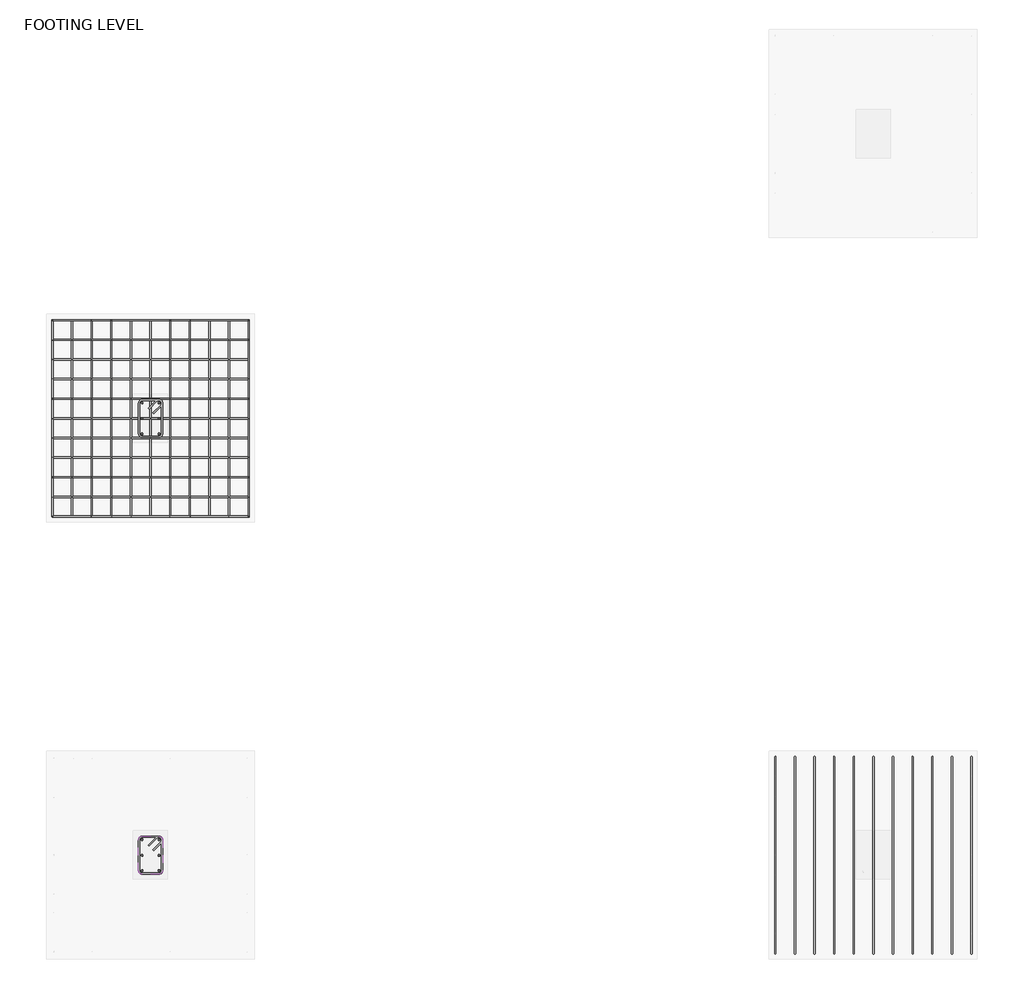
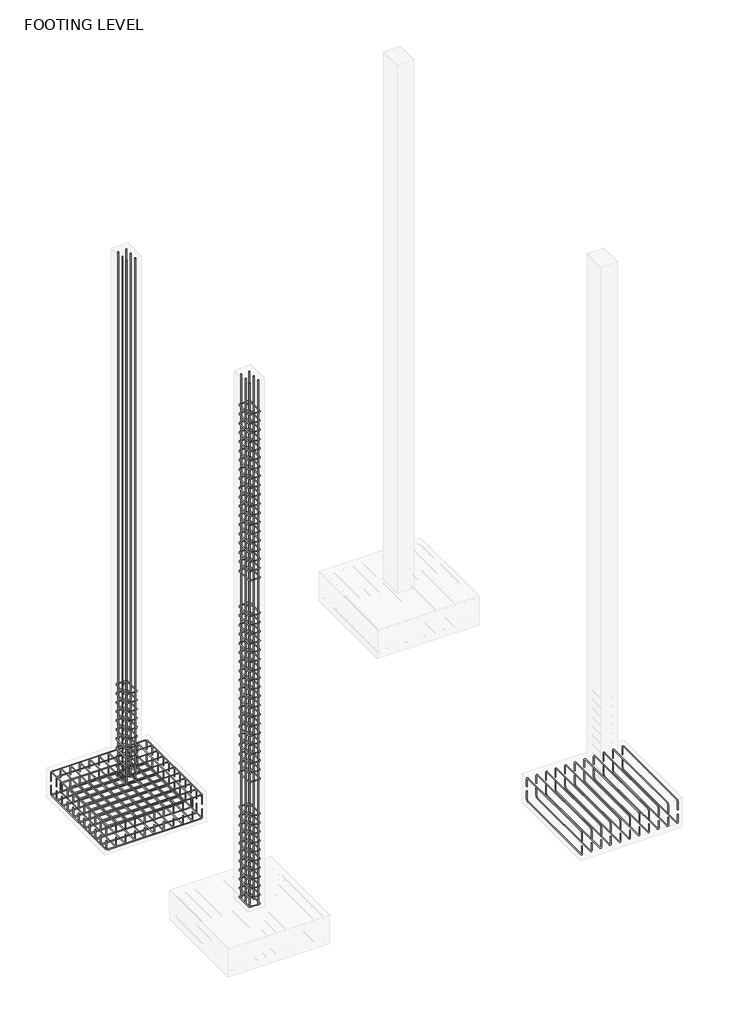
# One storey, part 3 of 9: 22 reinforcing bars.
"""IFC4 building model written with IfcOpenShell, lengths in millimetres."""

from ifc_helpers import new_model, si_unit, point, frame, origin, place, context, project, spatial, polyline, circle_curve, trimmed, segment, composite_curve, source, transform, mapped, element, save
from ifc_brep_helpers import swept_disk

model = new_model("IFC4")

# Units and contexts
model_context = context("Model", 3, world=origin())
ifc_project = project(units=[si_unit("LENGTHUNIT", "METRE", prefix="MILLI")], contexts=[model_context])

# Site, building, storey
site = spatial("IfcSite", under=ifc_project)
building = spatial("IfcBuilding", under=site)
storey = spatial("IfcBuildingStorey", under=building, Name="FOOTING LEVEL", Elevation=-1981.2)

# Reinforcing bars
placement = place(None, origin())
reinforcing_bar_shape = source(origin(), model_context, "Body", "SolidModel", [
    swept_disk(composite_curve([segment(polyline([(-2537.1816189, -3042.2841598, -2171.7), (-2537.1816189, -3042.2841598, -2057.4)]), True, "CONTINUOUS"), segment(trimmed(circle_curve(frame((-2537.1816189, -3075.6216598, -2057.4), z_axis=(1.0, 0.0, 0.0), x_axis=(0.0, 33.33750000000009, 0.0)), 33.3375), [point((-2537.1816189, -3042.2841598, -2057.4))], [point((-2537.1816189, -3075.6216598, -2024.0625))], True, "CARTESIAN"), True, "CONTINUOUS"), segment(polyline([(-2537.1816189, -3075.6216598, -2024.0625), (-2537.1816189, -4447.2216598, -2024.0625)]), True, "CONTINUOUS"), segment(trimmed(circle_curve(frame((-2537.1816189, -4447.2216598, -2057.4), z_axis=(1.0, 0.0, 0.0), x_axis=(0.0, 0.0, 33.33750000000009)), 33.3375), [point((-2537.1816189, -4447.2216598, -2024.0625))], [point((-2537.1816189, -4480.5591598, -2057.4))], True, "CARTESIAN"), True, "CONTINUOUS"), segment(polyline([(-2537.1816189, -4480.5591598, -2057.4), (-2537.1816189, -4480.5591598, -2171.7)]), True, "CONTINUOUS")], self_intersect=False), 4.7625),
])
element("IfcReinforcingBar", 1, at=placement, inside=storey, context=model_context, shape_type="MappedRepresentation", body=[
    mapped(reinforcing_bar_shape, transform((0.0, 0.0, 0.0), x_axis=(1.0, 0.0, 0.0), y_axis=(0.0, 1.0, 0.0), z_axis=(0.0, 0.0, 1.0))),
    mapped(reinforcing_bar_shape, transform((-143.8275, 0.0, 0.0), x_axis=(1.0, 0.0, 0.0), y_axis=(0.0, 1.0, 0.0), z_axis=(0.0, 0.0, 1.0))),
    mapped(reinforcing_bar_shape, transform((-287.655, 0.0, 0.0), x_axis=(1.0, 0.0, 0.0), y_axis=(0.0, 1.0, 0.0), z_axis=(0.0, 0.0, 1.0))),
    mapped(reinforcing_bar_shape, transform((-431.4825, 0.0, 0.0), x_axis=(1.0, 0.0, 0.0), y_axis=(0.0, 1.0, 0.0), z_axis=(0.0, 0.0, 1.0))),
    mapped(reinforcing_bar_shape, transform((-575.31, 0.0, 0.0), x_axis=(1.0, 0.0, 0.0), y_axis=(0.0, 1.0, 0.0), z_axis=(0.0, 0.0, 1.0))),
    mapped(reinforcing_bar_shape, transform((-719.1375, 0.0, 0.0), x_axis=(1.0, 0.0, 0.0), y_axis=(0.0, 1.0, 0.0), z_axis=(0.0, 0.0, 1.0))),
    mapped(reinforcing_bar_shape, transform((-862.965, 0.0, 0.0), x_axis=(1.0, 0.0, 0.0), y_axis=(0.0, 1.0, 0.0), z_axis=(0.0, 0.0, 1.0))),
    mapped(reinforcing_bar_shape, transform((-1006.7925, 0.0, 0.0), x_axis=(1.0, 0.0, 0.0), y_axis=(0.0, 1.0, 0.0), z_axis=(0.0, 0.0, 1.0))),
    mapped(reinforcing_bar_shape, transform((-1150.62, 0.0, 0.0), x_axis=(1.0, 0.0, 0.0), y_axis=(0.0, 1.0, 0.0), z_axis=(0.0, 0.0, 1.0))),
    mapped(reinforcing_bar_shape, transform((-1294.4475, 0.0, 0.0), x_axis=(1.0, 0.0, 0.0), y_axis=(0.0, 1.0, 0.0), z_axis=(0.0, 0.0, 1.0))),
    mapped(reinforcing_bar_shape, transform((-1438.275, 0.0, 0.0), x_axis=(1.0, 0.0, 0.0), y_axis=(0.0, 1.0, 0.0), z_axis=(0.0, 0.0, 1.0))),
])
reinforcing_bar_2_shape = source(origin(), model_context, "Body", "SolidModel", [
    swept_disk(composite_curve([segment(polyline([(-2537.1816189, -4480.5591598, -2247.9), (-2537.1816189, -4480.5591598, -2362.2)]), True, "CONTINUOUS"), segment(trimmed(circle_curve(frame((-2537.1816189, -4447.2216598, -2362.2), z_axis=(1.0, 0.0, 0.0), x_axis=(0.0, -33.337499999999636, 0.0)), 33.3375), [point((-2537.1816189, -4480.5591598, -2362.2))], [point((-2537.1816189, -4447.2216598, -2395.5375))], True, "CARTESIAN"), True, "CONTINUOUS"), segment(polyline([(-2537.1816189, -4447.2216598, -2395.5375), (-2537.1816189, -3075.6216598, -2395.5375)]), True, "CONTINUOUS"), segment(trimmed(circle_curve(frame((-2537.1816189, -3075.6216598, -2362.2), z_axis=(1.0, 0.0, 0.0), x_axis=(0.0, 0.0, -33.33750000000009)), 33.3375), [point((-2537.1816189, -3075.6216598, -2395.5375))], [point((-2537.1816189, -3042.2841598, -2362.2))], True, "CARTESIAN"), True, "CONTINUOUS"), segment(polyline([(-2537.1816189, -3042.2841598, -2362.2), (-2537.1816189, -3042.2841598, -2247.9)]), True, "CONTINUOUS")], self_intersect=False), 4.7625),
])
element("IfcReinforcingBar", 2, at=placement, inside=storey, context=model_context, shape_type="MappedRepresentation", body=[
    mapped(reinforcing_bar_2_shape, transform((0.0, 0.0, 0.0), x_axis=(1.0, 0.0, 0.0), y_axis=(0.0, 1.0, 0.0), z_axis=(0.0, 0.0, 1.0))),
    mapped(reinforcing_bar_2_shape, transform((-143.8275, 0.0, 0.0), x_axis=(1.0, 0.0, 0.0), y_axis=(0.0, 1.0, 0.0), z_axis=(0.0, 0.0, 1.0))),
    mapped(reinforcing_bar_2_shape, transform((-287.655, 0.0, 0.0), x_axis=(1.0, 0.0, 0.0), y_axis=(0.0, 1.0, 0.0), z_axis=(0.0, 0.0, 1.0))),
    mapped(reinforcing_bar_2_shape, transform((-431.4825, 0.0, 0.0), x_axis=(1.0, 0.0, 0.0), y_axis=(0.0, 1.0, 0.0), z_axis=(0.0, 0.0, 1.0))),
    mapped(reinforcing_bar_2_shape, transform((-575.31, 0.0, 0.0), x_axis=(1.0, 0.0, 0.0), y_axis=(0.0, 1.0, 0.0), z_axis=(0.0, 0.0, 1.0))),
    mapped(reinforcing_bar_2_shape, transform((-719.1375, 0.0, 0.0), x_axis=(1.0, 0.0, 0.0), y_axis=(0.0, 1.0, 0.0), z_axis=(0.0, 0.0, 1.0))),
    mapped(reinforcing_bar_2_shape, transform((-862.965, 0.0, 0.0), x_axis=(1.0, 0.0, 0.0), y_axis=(0.0, 1.0, 0.0), z_axis=(0.0, 0.0, 1.0))),
    mapped(reinforcing_bar_2_shape, transform((-1006.7925, 0.0, 0.0), x_axis=(1.0, 0.0, 0.0), y_axis=(0.0, 1.0, 0.0), z_axis=(0.0, 0.0, 1.0))),
    mapped(reinforcing_bar_2_shape, transform((-1150.62, 0.0, 0.0), x_axis=(1.0, 0.0, 0.0), y_axis=(0.0, 1.0, 0.0), z_axis=(0.0, 0.0, 1.0))),
    mapped(reinforcing_bar_2_shape, transform((-1294.4475, 0.0, 0.0), x_axis=(1.0, 0.0, 0.0), y_axis=(0.0, 1.0, 0.0), z_axis=(0.0, 0.0, 1.0))),
    mapped(reinforcing_bar_2_shape, transform((-1438.275, 0.0, 0.0), x_axis=(1.0, 0.0, 0.0), y_axis=(0.0, 1.0, 0.0), z_axis=(0.0, 0.0, 1.0))),
])
reinforcing_bar_3_shape = source(origin(), model_context, "Body", "SolidModel", [
    swept_disk(composite_curve([segment(polyline([(-7832.9458659, 158.1158402, -2171.7), (-7832.9458659, 158.1158402, -2057.4)]), True, "CONTINUOUS"), segment(trimmed(circle_curve(frame((-7832.9458659, 124.7783402, -2057.4), z_axis=(1.0, 0.0, 0.0), x_axis=(0.0, 33.337500000000006, 0.0)), 33.3375), [point((-7832.9458659, 158.1158402, -2057.4))], [point((-7832.9458659, 124.7783402, -2024.0625))], True, "CARTESIAN"), True, "CONTINUOUS"), segment(polyline([(-7832.9458659, 124.7783402, -2024.0625), (-7832.9458659, -1246.8216598, -2024.0625)]), True, "CONTINUOUS"), segment(trimmed(circle_curve(frame((-7832.9458659, -1246.8216598, -2057.4), z_axis=(1.0, 0.0, 0.0), x_axis=(0.0, 0.0, 33.33750000000009)), 33.3375), [point((-7832.9458659, -1246.8216598, -2024.0625))], [point((-7832.9458659, -1280.1591598, -2057.4))], True, "CARTESIAN"), True, "CONTINUOUS"), segment(polyline([(-7832.9458659, -1280.1591598, -2057.4), (-7832.9458659, -1280.1591598, -2171.7)]), True, "CONTINUOUS")], self_intersect=False), 4.7625),
])
element("IfcReinforcingBar", 3, at=placement, inside=storey, context=model_context, shape_type="MappedRepresentation", body=[
    mapped(reinforcing_bar_3_shape, transform((0.0, 0.0, 0.0), x_axis=(1.0, 0.0, 0.0), y_axis=(0.0, 1.0, 0.0), z_axis=(0.0, 0.0, 1.0))),
    mapped(reinforcing_bar_3_shape, transform((-143.8275, 0.0, 0.0), x_axis=(1.0, 0.0, 0.0), y_axis=(0.0, 1.0, 0.0), z_axis=(0.0, 0.0, 1.0))),
    mapped(reinforcing_bar_3_shape, transform((-287.655, 0.0, 0.0), x_axis=(1.0, 0.0, 0.0), y_axis=(0.0, 1.0, 0.0), z_axis=(0.0, 0.0, 1.0))),
    mapped(reinforcing_bar_3_shape, transform((-431.4825, 0.0, 0.0), x_axis=(1.0, 0.0, 0.0), y_axis=(0.0, 1.0, 0.0), z_axis=(0.0, 0.0, 1.0))),
    mapped(reinforcing_bar_3_shape, transform((-575.31, 0.0, 0.0), x_axis=(1.0, 0.0, 0.0), y_axis=(0.0, 1.0, 0.0), z_axis=(0.0, 0.0, 1.0))),
    mapped(reinforcing_bar_3_shape, transform((-719.1375, 0.0, 0.0), x_axis=(1.0, 0.0, 0.0), y_axis=(0.0, 1.0, 0.0), z_axis=(0.0, 0.0, 1.0))),
    mapped(reinforcing_bar_3_shape, transform((-862.965, 0.0, 0.0), x_axis=(1.0, 0.0, 0.0), y_axis=(0.0, 1.0, 0.0), z_axis=(0.0, 0.0, 1.0))),
    mapped(reinforcing_bar_3_shape, transform((-1006.7925, 0.0, 0.0), x_axis=(1.0, 0.0, 0.0), y_axis=(0.0, 1.0, 0.0), z_axis=(0.0, 0.0, 1.0))),
    mapped(reinforcing_bar_3_shape, transform((-1150.62, 0.0, 0.0), x_axis=(1.0, 0.0, 0.0), y_axis=(0.0, 1.0, 0.0), z_axis=(0.0, 0.0, 1.0))),
    mapped(reinforcing_bar_3_shape, transform((-1294.4475, 0.0, 0.0), x_axis=(1.0, 0.0, 0.0), y_axis=(0.0, 1.0, 0.0), z_axis=(0.0, 0.0, 1.0))),
    mapped(reinforcing_bar_3_shape, transform((-1438.275, 0.0, 0.0), x_axis=(1.0, 0.0, 0.0), y_axis=(0.0, 1.0, 0.0), z_axis=(0.0, 0.0, 1.0))),
])
reinforcing_bar_4_shape = source(origin(), model_context, "Body", "SolidModel", [
    swept_disk(composite_curve([segment(polyline([(-7832.9458659, -1280.1591598, -2247.9), (-7832.9458659, -1280.1591598, -2362.2)]), True, "CONTINUOUS"), segment(trimmed(circle_curve(frame((-7832.9458659, -1246.8216598, -2362.2), z_axis=(1.0, 0.0, 0.0), x_axis=(0.0, -33.33750000000009, 0.0)), 33.3375), [point((-7832.9458659, -1280.1591598, -2362.2))], [point((-7832.9458659, -1246.8216598, -2395.5375))], True, "CARTESIAN"), True, "CONTINUOUS"), segment(polyline([(-7832.9458659, -1246.8216598, -2395.5375), (-7832.9458659, 124.7783402, -2395.5375)]), True, "CONTINUOUS"), segment(trimmed(circle_curve(frame((-7832.9458659, 124.7783402, -2362.2), z_axis=(1.0, 0.0, 0.0), x_axis=(0.0, 0.0, -33.33750000000009)), 33.3375), [point((-7832.9458659, 124.7783402, -2395.5375))], [point((-7832.9458659, 158.1158402, -2362.2))], True, "CARTESIAN"), True, "CONTINUOUS"), segment(polyline([(-7832.9458659, 158.1158402, -2362.2), (-7832.9458659, 158.1158402, -2247.9)]), True, "CONTINUOUS")], self_intersect=False), 4.7625),
])
element("IfcReinforcingBar", 4, at=placement, inside=storey, context=model_context, shape_type="MappedRepresentation", body=[
    mapped(reinforcing_bar_4_shape, transform((0.0, 0.0, 0.0), x_axis=(1.0, 0.0, 0.0), y_axis=(0.0, 1.0, 0.0), z_axis=(0.0, 0.0, 1.0))),
    mapped(reinforcing_bar_4_shape, transform((-143.8275, 0.0, 0.0), x_axis=(1.0, 0.0, 0.0), y_axis=(0.0, 1.0, 0.0), z_axis=(0.0, 0.0, 1.0))),
    mapped(reinforcing_bar_4_shape, transform((-287.655, 0.0, 0.0), x_axis=(1.0, 0.0, 0.0), y_axis=(0.0, 1.0, 0.0), z_axis=(0.0, 0.0, 1.0))),
    mapped(reinforcing_bar_4_shape, transform((-431.4825, 0.0, 0.0), x_axis=(1.0, 0.0, 0.0), y_axis=(0.0, 1.0, 0.0), z_axis=(0.0, 0.0, 1.0))),
    mapped(reinforcing_bar_4_shape, transform((-575.31, 0.0, 0.0), x_axis=(1.0, 0.0, 0.0), y_axis=(0.0, 1.0, 0.0), z_axis=(0.0, 0.0, 1.0))),
    mapped(reinforcing_bar_4_shape, transform((-719.1375, 0.0, 0.0), x_axis=(1.0, 0.0, 0.0), y_axis=(0.0, 1.0, 0.0), z_axis=(0.0, 0.0, 1.0))),
    mapped(reinforcing_bar_4_shape, transform((-862.965, 0.0, 0.0), x_axis=(1.0, 0.0, 0.0), y_axis=(0.0, 1.0, 0.0), z_axis=(0.0, 0.0, 1.0))),
    mapped(reinforcing_bar_4_shape, transform((-1006.7925, 0.0, 0.0), x_axis=(1.0, 0.0, 0.0), y_axis=(0.0, 1.0, 0.0), z_axis=(0.0, 0.0, 1.0))),
    mapped(reinforcing_bar_4_shape, transform((-1150.62, 0.0, 0.0), x_axis=(1.0, 0.0, 0.0), y_axis=(0.0, 1.0, 0.0), z_axis=(0.0, 0.0, 1.0))),
    mapped(reinforcing_bar_4_shape, transform((-1294.4475, 0.0, 0.0), x_axis=(1.0, 0.0, 0.0), y_axis=(0.0, 1.0, 0.0), z_axis=(0.0, 0.0, 1.0))),
    mapped(reinforcing_bar_4_shape, transform((-1438.275, 0.0, 0.0), x_axis=(1.0, 0.0, 0.0), y_axis=(0.0, 1.0, 0.0), z_axis=(0.0, 0.0, 1.0))),
])
reinforcing_bar_5_shape = source(origin(), model_context, "Body", "SolidModel", [
    swept_disk(composite_curve([segment(polyline([(-9271.2208659, 158.1158402, -2171.7), (-9271.2208659, 158.1158402, -2057.4)]), True, "CONTINUOUS"), segment(trimmed(circle_curve(frame((-9237.8833659, 158.1158402, -2057.4), z_axis=(0.0, 1.0, 0.0), x_axis=(-33.337500000001455, 0.0, 0.0)), 33.3375), [point((-9271.2208659, 158.1158402, -2057.4))], [point((-9237.8833659, 158.1158402, -2024.0625))], True, "CARTESIAN"), True, "CONTINUOUS"), segment(polyline([(-9237.8833659, 158.1158402, -2024.0625), (-7866.2833659, 158.1158402, -2024.0625)]), True, "CONTINUOUS"), segment(trimmed(circle_curve(frame((-7866.2833659, 158.1158402, -2057.4), z_axis=(0.0, 1.0, 0.0), x_axis=(0.0, 0.0, 33.33750000000009)), 33.3375), [point((-7866.2833659, 158.1158402, -2024.0625))], [point((-7832.9458659, 158.1158402, -2057.4))], True, "CARTESIAN"), True, "CONTINUOUS"), segment(polyline([(-7832.9458659, 158.1158402, -2057.4), (-7832.9458659, 158.1158402, -2171.7)]), True, "CONTINUOUS")], self_intersect=False), 4.7625),
])
element("IfcReinforcingBar", 5, at=placement, inside=storey, context=model_context, shape_type="MappedRepresentation", body=[
    mapped(reinforcing_bar_5_shape, transform((0.0, 0.0, 0.0), x_axis=(1.0, 0.0, 0.0), y_axis=(0.0, 1.0, 0.0), z_axis=(0.0, 0.0, 1.0))),
    mapped(reinforcing_bar_5_shape, transform((0.0, -143.8275, 0.0), x_axis=(1.0, 0.0, 0.0), y_axis=(0.0, 1.0, 0.0), z_axis=(0.0, 0.0, 1.0))),
    mapped(reinforcing_bar_5_shape, transform((0.0, -287.655, 0.0), x_axis=(1.0, 0.0, 0.0), y_axis=(0.0, 1.0, 0.0), z_axis=(0.0, 0.0, 1.0))),
    mapped(reinforcing_bar_5_shape, transform((0.0, -431.4825, 0.0), x_axis=(1.0, 0.0, 0.0), y_axis=(0.0, 1.0, 0.0), z_axis=(0.0, 0.0, 1.0))),
    mapped(reinforcing_bar_5_shape, transform((0.0, -575.31, 0.0), x_axis=(1.0, 0.0, 0.0), y_axis=(0.0, 1.0, 0.0), z_axis=(0.0, 0.0, 1.0))),
    mapped(reinforcing_bar_5_shape, transform((0.0, -719.1375, 0.0), x_axis=(1.0, 0.0, 0.0), y_axis=(0.0, 1.0, 0.0), z_axis=(0.0, 0.0, 1.0))),
    mapped(reinforcing_bar_5_shape, transform((0.0, -862.965, 0.0), x_axis=(1.0, 0.0, 0.0), y_axis=(0.0, 1.0, 0.0), z_axis=(0.0, 0.0, 1.0))),
    mapped(reinforcing_bar_5_shape, transform((0.0, -1006.7925, 0.0), x_axis=(1.0, 0.0, 0.0), y_axis=(0.0, 1.0, 0.0), z_axis=(0.0, 0.0, 1.0))),
    mapped(reinforcing_bar_5_shape, transform((0.0, -1150.62, 0.0), x_axis=(1.0, 0.0, 0.0), y_axis=(0.0, 1.0, 0.0), z_axis=(0.0, 0.0, 1.0))),
    mapped(reinforcing_bar_5_shape, transform((0.0, -1294.4475, 0.0), x_axis=(1.0, 0.0, 0.0), y_axis=(0.0, 1.0, 0.0), z_axis=(0.0, 0.0, 1.0))),
    mapped(reinforcing_bar_5_shape, transform((0.0, -1438.275, 0.0), x_axis=(1.0, 0.0, 0.0), y_axis=(0.0, 1.0, 0.0), z_axis=(0.0, 0.0, 1.0))),
])
reinforcing_bar_6_shape = source(origin(), model_context, "Body", "SolidModel", [
    swept_disk(composite_curve([segment(polyline([(-9271.2208659, -1280.1591598, -2247.9), (-9271.2208659, -1280.1591598, -2362.2)]), True, "CONTINUOUS"), segment(trimmed(circle_curve(frame((-9237.8833659, -1280.1591598, -2362.2), z_axis=(0.0, -1.0, 0.0), x_axis=(-33.337500000001455, 0.0, 0.0)), 33.3375), [point((-9271.2208659, -1280.1591598, -2362.2))], [point((-9237.8833659, -1280.1591598, -2395.5375))], True, "CARTESIAN"), True, "CONTINUOUS"), segment(polyline([(-9237.8833659, -1280.1591598, -2395.5375), (-7866.2833659, -1280.1591598, -2395.5375)]), True, "CONTINUOUS"), segment(trimmed(circle_curve(frame((-7866.2833659, -1280.1591598, -2362.2), z_axis=(0.0, -1.0, 0.0), x_axis=(0.0, 0.0, -33.33750000000009)), 33.3375), [point((-7866.2833659, -1280.1591598, -2395.5375))], [point((-7832.9458659, -1280.1591598, -2362.2))], True, "CARTESIAN"), True, "CONTINUOUS"), segment(polyline([(-7832.9458659, -1280.1591598, -2362.2), (-7832.9458659, -1280.1591598, -2247.9)]), True, "CONTINUOUS")], self_intersect=False), 4.7625),
])
element("IfcReinforcingBar", 6, at=placement, inside=storey, context=model_context, shape_type="MappedRepresentation", body=[
    mapped(reinforcing_bar_6_shape, transform((0.0, 0.0, 0.0), x_axis=(1.0, 0.0, 0.0), y_axis=(0.0, 1.0, 0.0), z_axis=(0.0, 0.0, 1.0))),
    mapped(reinforcing_bar_6_shape, transform((0.0, 143.8275, 0.0), x_axis=(1.0, 0.0, 0.0), y_axis=(0.0, 1.0, 0.0), z_axis=(0.0, 0.0, 1.0))),
    mapped(reinforcing_bar_6_shape, transform((0.0, 287.655, 0.0), x_axis=(1.0, 0.0, 0.0), y_axis=(0.0, 1.0, 0.0), z_axis=(0.0, 0.0, 1.0))),
    mapped(reinforcing_bar_6_shape, transform((0.0, 431.4825, 0.0), x_axis=(1.0, 0.0, 0.0), y_axis=(0.0, 1.0, 0.0), z_axis=(0.0, 0.0, 1.0))),
    mapped(reinforcing_bar_6_shape, transform((0.0, 575.31, 0.0), x_axis=(1.0, 0.0, 0.0), y_axis=(0.0, 1.0, 0.0), z_axis=(0.0, 0.0, 1.0))),
    mapped(reinforcing_bar_6_shape, transform((0.0, 719.1375, 0.0), x_axis=(1.0, 0.0, 0.0), y_axis=(0.0, 1.0, 0.0), z_axis=(0.0, 0.0, 1.0))),
    mapped(reinforcing_bar_6_shape, transform((0.0, 862.965, 0.0), x_axis=(1.0, 0.0, 0.0), y_axis=(0.0, 1.0, 0.0), z_axis=(0.0, 0.0, 1.0))),
    mapped(reinforcing_bar_6_shape, transform((0.0, 1006.7925, 0.0), x_axis=(1.0, 0.0, 0.0), y_axis=(0.0, 1.0, 0.0), z_axis=(0.0, 0.0, 1.0))),
    mapped(reinforcing_bar_6_shape, transform((0.0, 1150.62, 0.0), x_axis=(1.0, 0.0, 0.0), y_axis=(0.0, 1.0, 0.0), z_axis=(0.0, 0.0, 1.0))),
    mapped(reinforcing_bar_6_shape, transform((0.0, 1294.4475, 0.0), x_axis=(1.0, 0.0, 0.0), y_axis=(0.0, 1.0, 0.0), z_axis=(0.0, 0.0, 1.0))),
    mapped(reinforcing_bar_6_shape, transform((0.0, 1438.275, 0.0), x_axis=(1.0, 0.0, 0.0), y_axis=(0.0, 1.0, 0.0), z_axis=(0.0, 0.0, 1.0))),
])
reinforcing_bar_7_shape = source(origin(), model_context, "Body", "SolidModel", [
    swept_disk(composite_curve([segment(polyline([(-8531.7845827, -523.5988371, -1938.3375), (-8474.9203857, -466.73464, -1938.3375)]), True, "CONTINUOUS"), segment(trimmed(circle_curve(frame((-8491.7583659, -449.8966598, -1938.3375), z_axis=(0.0, 0.0, 1.0), x_axis=(16.837980199999947, -16.837980200000004, 0.0)), 23.8125), [point((-8474.9203857, -466.73464, -1938.3375))], [point((-8491.7583659, -426.0841598, -1938.3375))], True, "CARTESIAN"), True, "CONTINUOUS"), segment(polyline([(-8491.7583659, -426.0841598, -1938.3375), (-8612.4083659, -426.0841598, -1938.3375)]), True, "CONTINUOUS"), segment(trimmed(circle_curve(frame((-8612.4083659, -449.8966598, -1938.3375), z_axis=(0.0, 0.0, 1.0), x_axis=(0.0, 23.8125, 0.0)), 23.8125), [point((-8612.4083659, -426.0841598, -1938.3375))], [point((-8636.2208659, -449.8966598, -1938.3375))], True, "CARTESIAN"), True, "CONTINUOUS"), segment(polyline([(-8636.2208659, -449.8966598, -1938.3375), (-8636.2208659, -672.1466598, -1938.3375)]), True, "CONTINUOUS"), segment(trimmed(circle_curve(frame((-8612.4464219, -672.1466598, -1939.6832232), z_axis=(0.056513312022656255, 0.0, 0.9984018457335854), x_axis=(-23.774444000000585, 0.0, 1.3457231999998385)), 23.8125), [point((-8636.2208659, -672.1466598, -1938.3375))], [point((-8612.4464219, -695.9591598, -1939.6832232))], True, "CARTESIAN"), True, "CONTINUOUS"), segment(polyline([(-8612.4464219, -695.9591598, -1939.6832232), (-8491.7203098, -695.9591598, -1946.5167768)]), True, "CONTINUOUS"), segment(trimmed(circle_curve(frame((-8491.7203098, -672.1466598, -1946.5167768), z_axis=(0.056513312022656255, 0.0, 0.9984018457335854), x_axis=(0.0, -23.8125, 0.0)), 23.8125), [point((-8491.7203098, -695.9591598, -1946.5167768))], [point((-8467.9458659, -672.1466598, -1947.8625))], True, "CARTESIAN"), True, "CONTINUOUS"), segment(polyline([(-8467.9458659, -672.1466598, -1947.8625), (-8467.9458659, -449.8966598, -1947.8625)]), True, "CONTINUOUS"), segment(trimmed(circle_curve(frame((-8491.7583659, -449.8966598, -1947.8625), z_axis=(0.0, 0.0, 1.0), x_axis=(23.8125, 0.0, 0.0)), 23.8125), [point((-8467.9458659, -449.8966598, -1947.8625))], [point((-8508.5963461, -433.0586796, -1947.8625))], True, "CARTESIAN"), True, "CONTINUOUS"), segment(polyline([(-8508.5963461, -433.0586796, -1947.8625), (-8565.4605432, -489.9228767, -1947.8625)]), True, "CONTINUOUS")], self_intersect=False), 4.7625),
])
element("IfcReinforcingBar", 7, at=placement, inside=storey, context=model_context, shape_type="MappedRepresentation", body=[
    mapped(reinforcing_bar_7_shape, transform((0.0, 0.0, 0.0), x_axis=(1.0, 0.0, 0.0), y_axis=(0.0, 1.0, 0.0), z_axis=(0.0, 0.0, 1.0))),
    mapped(reinforcing_bar_7_shape, transform((0.0, 0.0, 143.379777), x_axis=(1.0, 0.0, 0.0), y_axis=(0.0, 1.0, 0.0), z_axis=(0.0, 0.0, 1.0))),
    mapped(reinforcing_bar_7_shape, transform((0.0, 0.0, 286.759554), x_axis=(1.0, 0.0, 0.0), y_axis=(0.0, 1.0, 0.0), z_axis=(0.0, 0.0, 1.0))),
    mapped(reinforcing_bar_7_shape, transform((0.0, 0.0, 430.1393311), x_axis=(1.0, 0.0, 0.0), y_axis=(0.0, 1.0, 0.0), z_axis=(0.0, 0.0, 1.0))),
    mapped(reinforcing_bar_7_shape, transform((0.0, 0.0, 573.5191081), x_axis=(1.0, 0.0, 0.0), y_axis=(0.0, 1.0, 0.0), z_axis=(0.0, 0.0, 1.0))),
    mapped(reinforcing_bar_7_shape, transform((0.0, 0.0, 716.8988851), x_axis=(1.0, 0.0, 0.0), y_axis=(0.0, 1.0, 0.0), z_axis=(0.0, 0.0, 1.0))),
    mapped(reinforcing_bar_7_shape, transform((0.0, 0.0, 860.2786621), x_axis=(1.0, 0.0, 0.0), y_axis=(0.0, 1.0, 0.0), z_axis=(0.0, 0.0, 1.0))),
    mapped(reinforcing_bar_7_shape, transform((0.0, 0.0, 1003.6584392), x_axis=(1.0, 0.0, 0.0), y_axis=(0.0, 1.0, 0.0), z_axis=(0.0, 0.0, 1.0))),
    mapped(reinforcing_bar_7_shape, transform((0.0, 0.0, 1147.0382162), x_axis=(1.0, 0.0, 0.0), y_axis=(0.0, 1.0, 0.0), z_axis=(0.0, 0.0, 1.0))),
    mapped(reinforcing_bar_7_shape, transform((0.0, 0.0, 1290.4179932), x_axis=(1.0, 0.0, 0.0), y_axis=(0.0, 1.0, 0.0), z_axis=(0.0, 0.0, 1.0))),
    mapped(reinforcing_bar_7_shape, transform((0.0, 0.0, 1433.7977702), x_axis=(1.0, 0.0, 0.0), y_axis=(0.0, 1.0, 0.0), z_axis=(0.0, 0.0, 1.0))),
])
element("IfcReinforcingBar", 8, at=placement, inside=storey, context=model_context, shape_type="SolidModel", body=[
    swept_disk(composite_curve([segment(polyline([(-8490.2784581, -674.5029989, -1943.1), (-8490.2784581, -674.5029989, 6362.7)]), True, "CONTINUOUS")], self_intersect=False), 6.35),
])
element("IfcReinforcingBar", 9, at=placement, inside=storey, context=model_context, shape_type="SolidModel", body=[
    swept_disk(composite_curve([segment(polyline([(-8613.8882737, -674.5029989, -1943.1), (-8613.8882737, -674.5029989, 6362.7)]), True, "CONTINUOUS")], self_intersect=False), 6.35),
])
element("IfcReinforcingBar", 10, at=placement, inside=storey, context=model_context, shape_type="SolidModel", body=[
    swept_disk(composite_curve([segment(polyline([(-8490.2784581, -447.5403207, -1943.1), (-8490.2784581, -447.5403207, 6362.7)]), True, "CONTINUOUS")], self_intersect=False), 6.35),
])
element("IfcReinforcingBar", 11, at=placement, inside=storey, context=model_context, shape_type="SolidModel", body=[
    swept_disk(composite_curve([segment(polyline([(-8613.8882737, -447.5403207, -1943.1), (-8613.8882737, -447.5403207, 6362.7)]), True, "CONTINUOUS")], self_intersect=False), 6.35),
])
element("IfcReinforcingBar", 12, at=placement, inside=storey, context=model_context, shape_type="SolidModel", body=[
    swept_disk(composite_curve([segment(polyline([(-8490.2784581, -561.8403207, -1943.1), (-8490.2784581, -561.8403207, 6362.7)]), True, "CONTINUOUS")], self_intersect=False), 6.35),
])
element("IfcReinforcingBar", 13, at=placement, inside=storey, context=model_context, shape_type="SolidModel", body=[
    swept_disk(composite_curve([segment(polyline([(-8613.8882737, -561.8403207, -1943.1), (-8613.8882737, -561.8403207, 6362.7)]), True, "CONTINUOUS")], self_intersect=False), 6.35),
])
reinforcing_bar_8_shape = source(origin(), model_context, "Body", "SolidModel", [
    swept_disk(composite_curve([segment(polyline([(-8531.7845827, -3723.9988371, -1938.3375), (-8474.9203857, -3667.13464, -1938.3375)]), True, "CONTINUOUS"), segment(trimmed(circle_curve(frame((-8491.7583659, -3650.2966598, -1938.3375), z_axis=(0.0, 0.0, 1.0), x_axis=(16.837980199999947, -16.837980200000402, 0.0)), 23.8125), [point((-8474.9203857, -3667.13464, -1938.3375))], [point((-8491.7583659, -3626.4841598, -1938.3375))], True, "CARTESIAN"), True, "CONTINUOUS"), segment(polyline([(-8491.7583659, -3626.4841598, -1938.3375), (-8612.4083659, -3626.4841598, -1938.3375)]), True, "CONTINUOUS"), segment(trimmed(circle_curve(frame((-8612.4083659, -3650.2966598, -1938.3375), z_axis=(0.0, 0.0, 1.0), x_axis=(0.0, 23.8125, 0.0)), 23.8125), [point((-8612.4083659, -3626.4841598, -1938.3375))], [point((-8636.2208659, -3650.2966598, -1938.3375))], True, "CARTESIAN"), True, "CONTINUOUS"), segment(polyline([(-8636.2208659, -3650.2966598, -1938.3375), (-8636.2208659, -3872.5466598, -1938.3375)]), True, "CONTINUOUS"), segment(trimmed(circle_curve(frame((-8612.4464219, -3872.5466598, -1939.6832232), z_axis=(0.056513312022656255, 0.0, 0.9984018457335854), x_axis=(-23.774444000000585, 0.0, 1.3457231999998385)), 23.8125), [point((-8636.2208659, -3872.5466598, -1938.3375))], [point((-8612.4464219, -3896.3591598, -1939.6832232))], True, "CARTESIAN"), True, "CONTINUOUS"), segment(polyline([(-8612.4464219, -3896.3591598, -1939.6832232), (-8491.7203098, -3896.3591598, -1946.5167768)]), True, "CONTINUOUS"), segment(trimmed(circle_curve(frame((-8491.7203098, -3872.5466598, -1946.5167768), z_axis=(0.056513312022656255, 0.0, 0.9984018457335854), x_axis=(0.0, -23.8125, 0.0)), 23.8125), [point((-8491.7203098, -3896.3591598, -1946.5167768))], [point((-8467.9458659, -3872.5466598, -1947.8625))], True, "CARTESIAN"), True, "CONTINUOUS"), segment(polyline([(-8467.9458659, -3872.5466598, -1947.8625), (-8467.9458659, -3650.2966598, -1947.8625)]), True, "CONTINUOUS"), segment(trimmed(circle_curve(frame((-8491.7583659, -3650.2966598, -1947.8625), z_axis=(0.0, 0.0, 1.0), x_axis=(23.8125, 0.0, 0.0)), 23.8125), [point((-8467.9458659, -3650.2966598, -1947.8625))], [point((-8508.5963461, -3633.4586796, -1947.8625))], True, "CARTESIAN"), True, "CONTINUOUS"), segment(polyline([(-8508.5963461, -3633.4586796, -1947.8625), (-8565.4605432, -3690.3228767, -1947.8625)]), True, "CONTINUOUS")], self_intersect=False), 4.7625),
])
element("IfcReinforcingBar", 14, at=placement, inside=storey, context=model_context, shape_type="MappedRepresentation", body=[
    mapped(reinforcing_bar_8_shape, transform((0.0, 0.0, 0.0), x_axis=(1.0, 0.0, 0.0), y_axis=(0.0, 1.0, 0.0), z_axis=(0.0, 0.0, 1.0))),
    mapped(reinforcing_bar_8_shape, transform((0.0, 0.0, 142.9363281), x_axis=(1.0, 0.0, 0.0), y_axis=(0.0, 1.0, 0.0), z_axis=(0.0, 0.0, 1.0))),
    mapped(reinforcing_bar_8_shape, transform((0.0, 0.0, 285.8726562), x_axis=(1.0, 0.0, 0.0), y_axis=(0.0, 1.0, 0.0), z_axis=(0.0, 0.0, 1.0))),
    mapped(reinforcing_bar_8_shape, transform((0.0, 0.0, 428.8089844), x_axis=(1.0, 0.0, 0.0), y_axis=(0.0, 1.0, 0.0), z_axis=(0.0, 0.0, 1.0))),
    mapped(reinforcing_bar_8_shape, transform((0.0, 0.0, 571.7453125), x_axis=(1.0, 0.0, 0.0), y_axis=(0.0, 1.0, 0.0), z_axis=(0.0, 0.0, 1.0))),
    mapped(reinforcing_bar_8_shape, transform((0.0, 0.0, 714.6816406), x_axis=(1.0, 0.0, 0.0), y_axis=(0.0, 1.0, 0.0), z_axis=(0.0, 0.0, 1.0))),
    mapped(reinforcing_bar_8_shape, transform((0.0, 0.0, 857.6179687), x_axis=(1.0, 0.0, 0.0), y_axis=(0.0, 1.0, 0.0), z_axis=(0.0, 0.0, 1.0))),
    mapped(reinforcing_bar_8_shape, transform((0.0, 0.0, 1000.5542969), x_axis=(1.0, 0.0, 0.0), y_axis=(0.0, 1.0, 0.0), z_axis=(0.0, 0.0, 1.0))),
    mapped(reinforcing_bar_8_shape, transform((0.0, 0.0, 1143.490625), x_axis=(1.0, 0.0, 0.0), y_axis=(0.0, 1.0, 0.0), z_axis=(0.0, 0.0, 1.0))),
    mapped(reinforcing_bar_8_shape, transform((0.0, 0.0, 1286.4269531), x_axis=(1.0, 0.0, 0.0), y_axis=(0.0, 1.0, 0.0), z_axis=(0.0, 0.0, 1.0))),
    mapped(reinforcing_bar_8_shape, transform((0.0, 0.0, 1429.3632812), x_axis=(1.0, 0.0, 0.0), y_axis=(0.0, 1.0, 0.0), z_axis=(0.0, 0.0, 1.0))),
])
element("IfcReinforcingBar", 15, at=placement, inside=storey, context=model_context, shape_type="SolidModel", body=[
    swept_disk(composite_curve([segment(polyline([(-8490.2784581, -3874.9029989, -1943.1), (-8490.2784581, -3874.9029989, 6362.7)]), True, "CONTINUOUS")], self_intersect=False), 6.35),
])
element("IfcReinforcingBar", 16, at=placement, inside=storey, context=model_context, shape_type="SolidModel", body=[
    swept_disk(composite_curve([segment(polyline([(-8613.8882737, -3874.9029989, -1943.1), (-8613.8882737, -3874.9029989, 6362.7)]), True, "CONTINUOUS")], self_intersect=False), 6.35),
])
element("IfcReinforcingBar", 17, at=placement, inside=storey, context=model_context, shape_type="SolidModel", body=[
    swept_disk(composite_curve([segment(polyline([(-8490.2784581, -3647.9403207, -1943.1), (-8490.2784581, -3647.9403207, 6362.7)]), True, "CONTINUOUS")], self_intersect=False), 6.35),
])
element("IfcReinforcingBar", 18, at=placement, inside=storey, context=model_context, shape_type="SolidModel", body=[
    swept_disk(composite_curve([segment(polyline([(-8613.8882737, -3647.9403207, -1943.1), (-8613.8882737, -3647.9403207, 6362.7)]), True, "CONTINUOUS")], self_intersect=False), 6.35),
])
element("IfcReinforcingBar", 19, at=placement, inside=storey, context=model_context, shape_type="SolidModel", body=[
    swept_disk(composite_curve([segment(polyline([(-8490.2784581, -3762.2403207, -1943.1), (-8490.2784581, -3762.2403207, 6362.7)]), True, "CONTINUOUS")], self_intersect=False), 6.35),
])
element("IfcReinforcingBar", 20, at=placement, inside=storey, context=model_context, shape_type="SolidModel", body=[
    swept_disk(composite_curve([segment(polyline([(-8613.8882737, -3762.2403207, -1943.1), (-8613.8882737, -3762.2403207, 6362.7)]), True, "CONTINUOUS")], self_intersect=False), 6.35),
])
reinforcing_bar_9_shape = source(origin(), model_context, "Body", "SolidModel", [
    swept_disk(composite_curve([segment(polyline([(-8531.7845827, -3723.9988371, 42.8625), (-8474.9203857, -3667.13464, 42.8625)]), True, "CONTINUOUS"), segment(trimmed(circle_curve(frame((-8491.7583659, -3650.2966598, 42.8625), z_axis=(0.0, 0.0, 1.0), x_axis=(16.837980199999947, -16.837980200000402, 0.0)), 23.8125), [point((-8474.9203857, -3667.13464, 42.8625))], [point((-8491.7583659, -3626.4841598, 42.8625))], True, "CARTESIAN"), True, "CONTINUOUS"), segment(polyline([(-8491.7583659, -3626.4841598, 42.8625), (-8612.4083659, -3626.4841598, 42.8625)]), True, "CONTINUOUS"), segment(trimmed(circle_curve(frame((-8612.4083659, -3650.2966598, 42.8625), z_axis=(0.0, 0.0, 1.0), x_axis=(0.0, 23.8125, 0.0)), 23.8125), [point((-8612.4083659, -3626.4841598, 42.8625))], [point((-8636.2208659, -3650.2966598, 42.8625))], True, "CARTESIAN"), True, "CONTINUOUS"), segment(polyline([(-8636.2208659, -3650.2966598, 42.8625), (-8636.2208659, -3872.5466598, 42.8625)]), True, "CONTINUOUS"), segment(trimmed(circle_curve(frame((-8612.4464219, -3872.5466598, 41.5167768), z_axis=(0.056513312022656255, 0.0, 0.9984018457335854), x_axis=(-23.774444000000585, 0.0, 1.3457231999999948)), 23.8125), [point((-8636.2208659, -3872.5466598, 42.8625))], [point((-8612.4464219, -3896.3591598, 41.5167768))], True, "CARTESIAN"), True, "CONTINUOUS"), segment(polyline([(-8612.4464219, -3896.3591598, 41.5167768), (-8491.7203098, -3896.3591598, 34.6832232)]), True, "CONTINUOUS"), segment(trimmed(circle_curve(frame((-8491.7203098, -3872.5466598, 34.6832232), z_axis=(0.056513312022656255, 0.0, 0.9984018457335854), x_axis=(0.0, -23.8125, 0.0)), 23.8125), [point((-8491.7203098, -3896.3591598, 34.6832232))], [point((-8467.9458659, -3872.5466598, 33.3375))], True, "CARTESIAN"), True, "CONTINUOUS"), segment(polyline([(-8467.9458659, -3872.5466598, 33.3375), (-8467.9458659, -3650.2966598, 33.3375)]), True, "CONTINUOUS"), segment(trimmed(circle_curve(frame((-8491.7583659, -3650.2966598, 33.3375), z_axis=(0.0, 0.0, 1.0), x_axis=(23.8125, 0.0, 0.0)), 23.8125), [point((-8467.9458659, -3650.2966598, 33.3375))], [point((-8508.5963461, -3633.4586796, 33.3375))], True, "CARTESIAN"), True, "CONTINUOUS"), segment(polyline([(-8508.5963461, -3633.4586796, 33.3375), (-8565.4605432, -3690.3228767, 33.3375)]), True, "CONTINUOUS")], self_intersect=False), 4.7625),
])
element("IfcReinforcingBar", 21, at=placement, inside=storey, context=model_context, shape_type="MappedRepresentation", body=[
    mapped(reinforcing_bar_9_shape, transform((0.0, 0.0, 0.0), x_axis=(1.0, 0.0, 0.0), y_axis=(0.0, 1.0, 0.0), z_axis=(0.0, 0.0, 1.0))),
    mapped(reinforcing_bar_9_shape, transform((0.0, 0.0, 146.3515264), x_axis=(1.0, 0.0, 0.0), y_axis=(0.0, 1.0, 0.0), z_axis=(0.0, 0.0, 1.0))),
    mapped(reinforcing_bar_9_shape, transform((0.0, 0.0, 292.7030529), x_axis=(1.0, 0.0, 0.0), y_axis=(0.0, 1.0, 0.0), z_axis=(0.0, 0.0, 1.0))),
    mapped(reinforcing_bar_9_shape, transform((0.0, 0.0, 439.0545793), x_axis=(1.0, 0.0, 0.0), y_axis=(0.0, 1.0, 0.0), z_axis=(0.0, 0.0, 1.0))),
    mapped(reinforcing_bar_9_shape, transform((0.0, 0.0, 585.4061058), x_axis=(1.0, 0.0, 0.0), y_axis=(0.0, 1.0, 0.0), z_axis=(0.0, 0.0, 1.0))),
    mapped(reinforcing_bar_9_shape, transform((0.0, 0.0, 731.7576322), x_axis=(1.0, 0.0, 0.0), y_axis=(0.0, 1.0, 0.0), z_axis=(0.0, 0.0, 1.0))),
    mapped(reinforcing_bar_9_shape, transform((0.0, 0.0, 878.1091586), x_axis=(1.0, 0.0, 0.0), y_axis=(0.0, 1.0, 0.0), z_axis=(0.0, 0.0, 1.0))),
    mapped(reinforcing_bar_9_shape, transform((0.0, 0.0, 1024.4606851), x_axis=(1.0, 0.0, 0.0), y_axis=(0.0, 1.0, 0.0), z_axis=(0.0, 0.0, 1.0))),
    mapped(reinforcing_bar_9_shape, transform((0.0, 0.0, 1170.8122115), x_axis=(1.0, 0.0, 0.0), y_axis=(0.0, 1.0, 0.0), z_axis=(0.0, 0.0, 1.0))),
    mapped(reinforcing_bar_9_shape, transform((0.0, 0.0, 1317.163738), x_axis=(1.0, 0.0, 0.0), y_axis=(0.0, 1.0, 0.0), z_axis=(0.0, 0.0, 1.0))),
    mapped(reinforcing_bar_9_shape, transform((0.0, 0.0, 1463.5152644), x_axis=(1.0, 0.0, 0.0), y_axis=(0.0, 1.0, 0.0), z_axis=(0.0, 0.0, 1.0))),
    mapped(reinforcing_bar_9_shape, transform((0.0, 0.0, 1609.8667908), x_axis=(1.0, 0.0, 0.0), y_axis=(0.0, 1.0, 0.0), z_axis=(0.0, 0.0, 1.0))),
    mapped(reinforcing_bar_9_shape, transform((0.0, 0.0, 1756.2183173), x_axis=(1.0, 0.0, 0.0), y_axis=(0.0, 1.0, 0.0), z_axis=(0.0, 0.0, 1.0))),
    mapped(reinforcing_bar_9_shape, transform((0.0, 0.0, 1902.5698437), x_axis=(1.0, 0.0, 0.0), y_axis=(0.0, 1.0, 0.0), z_axis=(0.0, 0.0, 1.0))),
    mapped(reinforcing_bar_9_shape, transform((0.0, 0.0, 2048.9213702), x_axis=(1.0, 0.0, 0.0), y_axis=(0.0, 1.0, 0.0), z_axis=(0.0, 0.0, 1.0))),
    mapped(reinforcing_bar_9_shape, transform((0.0, 0.0, 2195.2728966), x_axis=(1.0, 0.0, 0.0), y_axis=(0.0, 1.0, 0.0), z_axis=(0.0, 0.0, 1.0))),
    mapped(reinforcing_bar_9_shape, transform((0.0, 0.0, 2341.6244231), x_axis=(1.0, 0.0, 0.0), y_axis=(0.0, 1.0, 0.0), z_axis=(0.0, 0.0, 1.0))),
    mapped(reinforcing_bar_9_shape, transform((0.0, 0.0, 2487.9759495), x_axis=(1.0, 0.0, 0.0), y_axis=(0.0, 1.0, 0.0), z_axis=(0.0, 0.0, 1.0))),
    mapped(reinforcing_bar_9_shape, transform((0.0, 0.0, 2634.3274759), x_axis=(1.0, 0.0, 0.0), y_axis=(0.0, 1.0, 0.0), z_axis=(0.0, 0.0, 1.0))),
])
reinforcing_bar_10_shape = source(origin(), model_context, "Body", "SolidModel", [
    swept_disk(composite_curve([segment(polyline([(-8531.7845827, -3723.9988371, 3243.2625), (-8474.9203857, -3667.13464, 3243.2625)]), True, "CONTINUOUS"), segment(trimmed(circle_curve(frame((-8491.7583659, -3650.2966598, 3243.2625), z_axis=(0.0, 0.0, 1.0), x_axis=(16.837980199999947, -16.837980200000402, 0.0)), 23.8125), [point((-8474.9203857, -3667.13464, 3243.2625))], [point((-8491.7583659, -3626.4841598, 3243.2625))], True, "CARTESIAN"), True, "CONTINUOUS"), segment(polyline([(-8491.7583659, -3626.4841598, 3243.2625), (-8612.4083659, -3626.4841598, 3243.2625)]), True, "CONTINUOUS"), segment(trimmed(circle_curve(frame((-8612.4083659, -3650.2966598, 3243.2625), z_axis=(0.0, 0.0, 1.0), x_axis=(0.0, 23.8125, 0.0)), 23.8125), [point((-8612.4083659, -3626.4841598, 3243.2625))], [point((-8636.2208659, -3650.2966598, 3243.2625))], True, "CARTESIAN"), True, "CONTINUOUS"), segment(polyline([(-8636.2208659, -3650.2966598, 3243.2625), (-8636.2208659, -3872.5466598, 3243.2625)]), True, "CONTINUOUS"), segment(trimmed(circle_curve(frame((-8612.4464219, -3872.5466598, 3241.9167768), z_axis=(0.056513312022656255, 0.0, 0.9984018457335854), x_axis=(-23.774444000000585, 0.0, 1.345723199999611)), 23.8125), [point((-8636.2208659, -3872.5466598, 3243.2625))], [point((-8612.4464219, -3896.3591598, 3241.9167768))], True, "CARTESIAN"), True, "CONTINUOUS"), segment(polyline([(-8612.4464219, -3896.3591598, 3241.9167768), (-8491.7203098, -3896.3591598, 3235.0832232)]), True, "CONTINUOUS"), segment(trimmed(circle_curve(frame((-8491.7203098, -3872.5466598, 3235.0832232), z_axis=(0.056513312022656255, 0.0, 0.9984018457335854), x_axis=(0.0, -23.8125, 0.0)), 23.8125), [point((-8491.7203098, -3896.3591598, 3235.0832232))], [point((-8467.9458659, -3872.5466598, 3233.7375))], True, "CARTESIAN"), True, "CONTINUOUS"), segment(polyline([(-8467.9458659, -3872.5466598, 3233.7375), (-8467.9458659, -3650.2966598, 3233.7375)]), True, "CONTINUOUS"), segment(trimmed(circle_curve(frame((-8491.7583659, -3650.2966598, 3233.7375), z_axis=(0.0, 0.0, 1.0), x_axis=(23.8125, 0.0, 0.0)), 23.8125), [point((-8467.9458659, -3650.2966598, 3233.7375))], [point((-8508.5963461, -3633.4586796, 3233.7375))], True, "CARTESIAN"), True, "CONTINUOUS"), segment(polyline([(-8508.5963461, -3633.4586796, 3233.7375), (-8565.4605432, -3690.3228767, 3233.7375)]), True, "CONTINUOUS")], self_intersect=False), 4.7625),
])
element("IfcReinforcingBar", 22, at=placement, inside=storey, context=model_context, shape_type="MappedRepresentation", body=[
    mapped(reinforcing_bar_10_shape, transform((0.0, 0.0, 0.0), x_axis=(1.0, 0.0, 0.0), y_axis=(0.0, 1.0, 0.0), z_axis=(0.0, 0.0, 1.0))),
    mapped(reinforcing_bar_10_shape, transform((0.0, 0.0, 146.3443085), x_axis=(1.0, 0.0, 0.0), y_axis=(0.0, 1.0, 0.0), z_axis=(0.0, 0.0, 1.0))),
    mapped(reinforcing_bar_10_shape, transform((0.0, 0.0, 292.688617), x_axis=(1.0, 0.0, 0.0), y_axis=(0.0, 1.0, 0.0), z_axis=(0.0, 0.0, 1.0))),
    mapped(reinforcing_bar_10_shape, transform((0.0, 0.0, 439.0329255), x_axis=(1.0, 0.0, 0.0), y_axis=(0.0, 1.0, 0.0), z_axis=(0.0, 0.0, 1.0))),
    mapped(reinforcing_bar_10_shape, transform((0.0, 0.0, 585.377234), x_axis=(1.0, 0.0, 0.0), y_axis=(0.0, 1.0, 0.0), z_axis=(0.0, 0.0, 1.0))),
    mapped(reinforcing_bar_10_shape, transform((0.0, 0.0, 731.7215426), x_axis=(1.0, 0.0, 0.0), y_axis=(0.0, 1.0, 0.0), z_axis=(0.0, 0.0, 1.0))),
    mapped(reinforcing_bar_10_shape, transform((0.0, 0.0, 878.0658511), x_axis=(1.0, 0.0, 0.0), y_axis=(0.0, 1.0, 0.0), z_axis=(0.0, 0.0, 1.0))),
    mapped(reinforcing_bar_10_shape, transform((0.0, 0.0, 1024.4101596), x_axis=(1.0, 0.0, 0.0), y_axis=(0.0, 1.0, 0.0), z_axis=(0.0, 0.0, 1.0))),
    mapped(reinforcing_bar_10_shape, transform((0.0, 0.0, 1170.7544681), x_axis=(1.0, 0.0, 0.0), y_axis=(0.0, 1.0, 0.0), z_axis=(0.0, 0.0, 1.0))),
    mapped(reinforcing_bar_10_shape, transform((0.0, 0.0, 1317.0987766), x_axis=(1.0, 0.0, 0.0), y_axis=(0.0, 1.0, 0.0), z_axis=(0.0, 0.0, 1.0))),
    mapped(reinforcing_bar_10_shape, transform((0.0, 0.0, 1463.4430851), x_axis=(1.0, 0.0, 0.0), y_axis=(0.0, 1.0, 0.0), z_axis=(0.0, 0.0, 1.0))),
    mapped(reinforcing_bar_10_shape, transform((0.0, 0.0, 1609.7873936), x_axis=(1.0, 0.0, 0.0), y_axis=(0.0, 1.0, 0.0), z_axis=(0.0, 0.0, 1.0))),
    mapped(reinforcing_bar_10_shape, transform((0.0, 0.0, 1756.1317021), x_axis=(1.0, 0.0, 0.0), y_axis=(0.0, 1.0, 0.0), z_axis=(0.0, 0.0, 1.0))),
    mapped(reinforcing_bar_10_shape, transform((0.0, 0.0, 1902.4760106), x_axis=(1.0, 0.0, 0.0), y_axis=(0.0, 1.0, 0.0), z_axis=(0.0, 0.0, 1.0))),
    mapped(reinforcing_bar_10_shape, transform((0.0, 0.0, 2048.8203192), x_axis=(1.0, 0.0, 0.0), y_axis=(0.0, 1.0, 0.0), z_axis=(0.0, 0.0, 1.0))),
    mapped(reinforcing_bar_10_shape, transform((0.0, 0.0, 2195.1646277), x_axis=(1.0, 0.0, 0.0), y_axis=(0.0, 1.0, 0.0), z_axis=(0.0, 0.0, 1.0))),
    mapped(reinforcing_bar_10_shape, transform((0.0, 0.0, 2341.5089362), x_axis=(1.0, 0.0, 0.0), y_axis=(0.0, 1.0, 0.0), z_axis=(0.0, 0.0, 1.0))),
    mapped(reinforcing_bar_10_shape, transform((0.0, 0.0, 2487.8532447), x_axis=(1.0, 0.0, 0.0), y_axis=(0.0, 1.0, 0.0), z_axis=(0.0, 0.0, 1.0))),
    mapped(reinforcing_bar_10_shape, transform((0.0, 0.0, 2634.1975532), x_axis=(1.0, 0.0, 0.0), y_axis=(0.0, 1.0, 0.0), z_axis=(0.0, 0.0, 1.0))),
])

save(model, "model.ifc")

# Revit data of these elements
# Elements 1, 2, 3, 4, 5, 6, 7, 8, 9, 10, 11, 12, 13, 14, 15, 16, 17, 18, 19, 20, 21, 22 (IfcReinforcingBar)
#   Phase Created = New Construction
